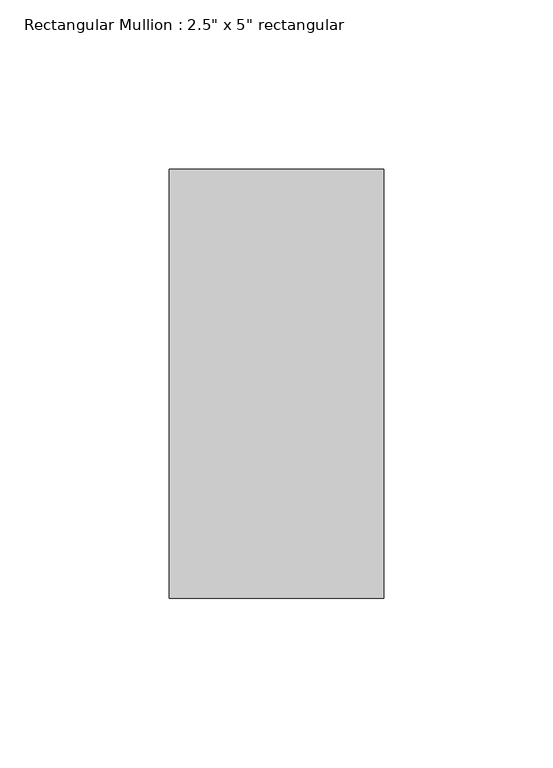
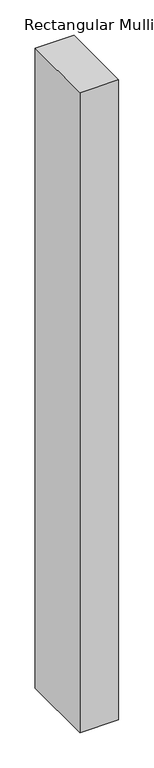
"""IFC4 building model written with IfcOpenShell, lengths in millimetres: member geometry."""

from ifc_helpers import new_model, si_unit, frame, origin, place, context, project, spatial, polyline, outline, extrude, source, transform, mapped, element, save


def member_3eefc08a(model_context):
    return source(origin(), model_context, "Body", "SweptSolid", [
        extrude(outline(polyline([(31.75, 63.5), (31.75, -63.5), (-31.75, -63.5), (-31.75, 63.5), (31.75, 63.5)])), frame((0.0, 0.0, -1106.2807647), z_axis=(0.0, 0.0, 1.0), x_axis=(1.0, 0.0, 0.0)), (0.0, 0.0, 1.0), 1106.2807647),
    ])


if __name__ == "__main__":
    model = new_model("IFC4")
    model_context = context("Model", 3, world=origin())
    ifc_project = project(units=[si_unit("LENGTHUNIT", "METRE", prefix="MILLI")], contexts=[model_context])
    site = spatial("IfcSite", under=ifc_project)
    building = spatial("IfcBuilding", under=site)
    placement = place(None, origin())
    member_shape = member_3eefc08a(model_context)
    element("IfcMember", 1, ObjectType="Rectangular Mullion : 2.5\" x 5\" rectangular", at=placement, inside=building, context=model_context, shape_type="MappedRepresentation", body=[
        mapped(member_shape, transform((0.0, 0.0, 0.0), x_axis=(1.0, 0.0, 0.0), y_axis=(0.0, 1.0, 0.0), z_axis=(0.0, 0.0, 1.0))),
    ])
    save(model, "model.ifc")

# Revit data of these elements
# Type "Rectangular Mullion : 2.5\" x 5\" rectangular"
#   built-in parameter 1007304 = 0.416667 (stored number, unit not read)
#   built-in parameter 1007301 = 0.104167 (stored number, unit not read)
#   built-in parameter 1007300 = 0.104167 (stored number, unit not read)
# Element 1 (IfcMember, "Rectangular Mullion : 2.5\" x 5\" rectangular")
#   Materials on its faces: "Aluminum"
# Materials
#   "Aluminum": class "Metal", colour RGB 247 247 247, transparency 0, Description = "Aluminum 6061", Cost = 0
